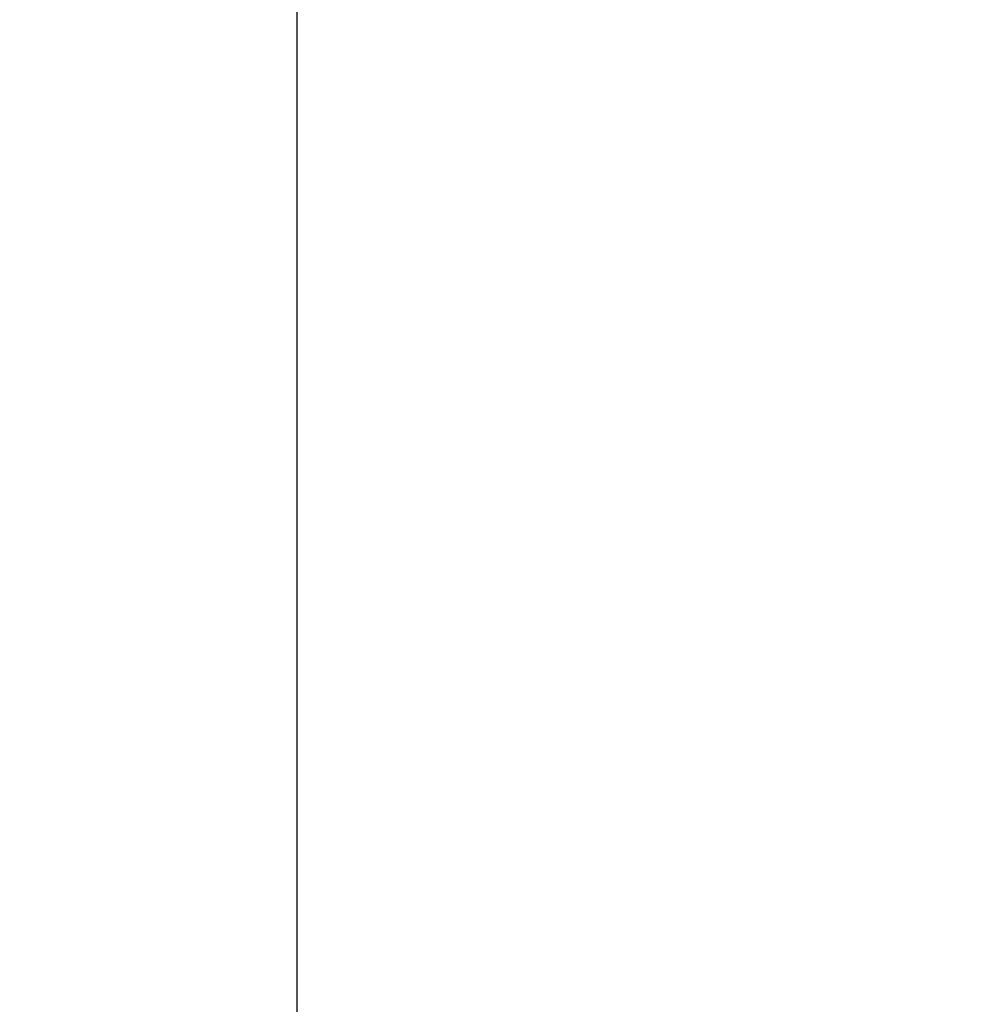
# Model space of a CAD drawing. Units: inches. Extents: x 2696 to 3240, y 1564 to 2310.
# Tile 10 of 76: x 2903.397 to 2912.112, y 1643.56 to 1652.487. Entities that reach past the tile are written whole.
import ezdxf

# ---------------------------------------------------------------- set-up
doc = ezdxf.new("R2010")
doc.units = ezdxf.units.IN
doc.layers.add('A-ANNO-DIMS', color=3, linetype='Continuous', lineweight=18)
doc.styles.add('TIMES NEW', font='times.ttf')
doc.dimstyles.new('Siddhuu', dxfattribs={"dimtxt": 6, "dimasz": 2.5, "dimexe": 1.25, "dimexo": 0.625, "dimtad": 1, "dimdec": 1, "dimlunit": 4, "dimtxsty": 'TIMES NEW', "dimcen": 2.5, "dimclrd": 256, "dimclre": 1, "dimclrt": 7, "dimadec": 0, "dimazin": 0, "dimtfac": 1, "dimtdec": 1, "dimtmove": 0, "dimatfit": 3, "dimfxl": 1, "dimtolj": 1, "dimlwd": -1, "dimarcsym": 0})

# ---------------------------------------------------------------- blocks, each defined once
blk = doc.blocks.new('*D57')
at = {"layer": 'A-ANNO-DIMS', "color": 1, "lineweight": -2, "transparency": 16777216}
for p, q in [((2754.6114, 2018.5761), (2754.6114, 1568.9511)), ((2956.7088, 2018.5761), (2956.7088, 1568.9511))]:
    blk.add_line(p, q, dxfattribs=at)
at = {"layer": 'A-ANNO-DIMS', "transparency": 16777216}
blk.add_line((2757.1114, 1570.2011), (2954.2088, 1570.2011), dxfattribs=at)
for points in [[(2757.1114, 1570.6178), (2757.1114, 1569.7844), (2754.6114, 1570.2011)], [(2954.2088, 1570.6178), (2954.2088, 1569.7844), (2956.7088, 1570.2011)]]:
    blk.add_solid(points, dxfattribs=at)
at = {"layer": 'Defpoints', "color": 0, "transparency": 16777216}
for p in [(2754.6114, 2019.2011), (2956.7088, 2019.2011), (2956.7088, 1570.2011)]:
    blk.add_point(p, dxfattribs=at)
at = {"layer": 'A-ANNO-DIMS', "color": 7, "transparency": 16777216, "insert": (2855.6601, 1573.878), "char_height": 6, "attachment_point": 5, "style": 'TIMES NEW'}
blk.add_mtext('\\A1;16\'-10"', dxfattribs=at)
blk = doc.blocks.new('*D69')
at = {"layer": 'A-ANNO-DIMS', "color": 1, "lineweight": -2, "transparency": 16777216}
for p, q in [((2841.889, 2261.5761), (2841.889, 1568.9511)), ((2905.9101, 2261.5761), (2905.9101, 1568.9511))]:
    blk.add_line(p, q, dxfattribs=at)
at = {"layer": 'A-ANNO-DIMS', "transparency": 16777216}
blk.add_line((2844.389, 1570.2011), (2903.4101, 1570.2011), dxfattribs=at)
for points in [[(2844.389, 1570.6178), (2844.389, 1569.7844), (2841.889, 1570.2011)], [(2903.4101, 1570.6178), (2903.4101, 1569.7844), (2905.9101, 1570.2011)]]:
    blk.add_solid(points, dxfattribs=at)
at = {"layer": 'Defpoints', "color": 0, "transparency": 16777216}
for p in [(2841.889, 2262.2011), (2905.9101, 2262.2011), (2905.9101, 1570.2011)]:
    blk.add_point(p, dxfattribs=at)
at = {"layer": 'A-ANNO-DIMS', "color": 7, "transparency": 16777216, "insert": (2873.8995, 1573.878), "char_height": 6, "attachment_point": 5, "style": 'TIMES NEW'}
blk.add_mtext('\\A1;5\'-4"', dxfattribs=at)

msp = doc.modelspace()

# ---------------------------------------------------------------- dimensions: what is measured, and where the dimension line sits
at = {"layer": 'A-ANNO-DIMS'}
for base, p1, p2, picture, middle in [((2905.9101, 1570.2011), (2841.889, 2262.2011), (2905.9101, 2262.2011), '*D69', (2873.8995, 1573.878)), ((2956.7088, 1570.2011), (2754.6114, 2019.2011), (2956.7088, 2019.2011), '*D57', (2855.6601, 1573.878))]:
    dim = msp.add_linear_dim(base=base, p1=p1, p2=p2, dimstyle='Siddhuu', override={"dimdec": 1, "dimlfac": 1, "dimrnd": 0, "dimzin": 1, "dimdsep": 46, "dimlunit": 4, "dimfrac": 2}, dxfattribs=at)
    dim.commit()
    dim.dimension.update_dxf_attribs({"geometry": picture, "text_midpoint": middle})

doc.saveas('drawing.dxf')
